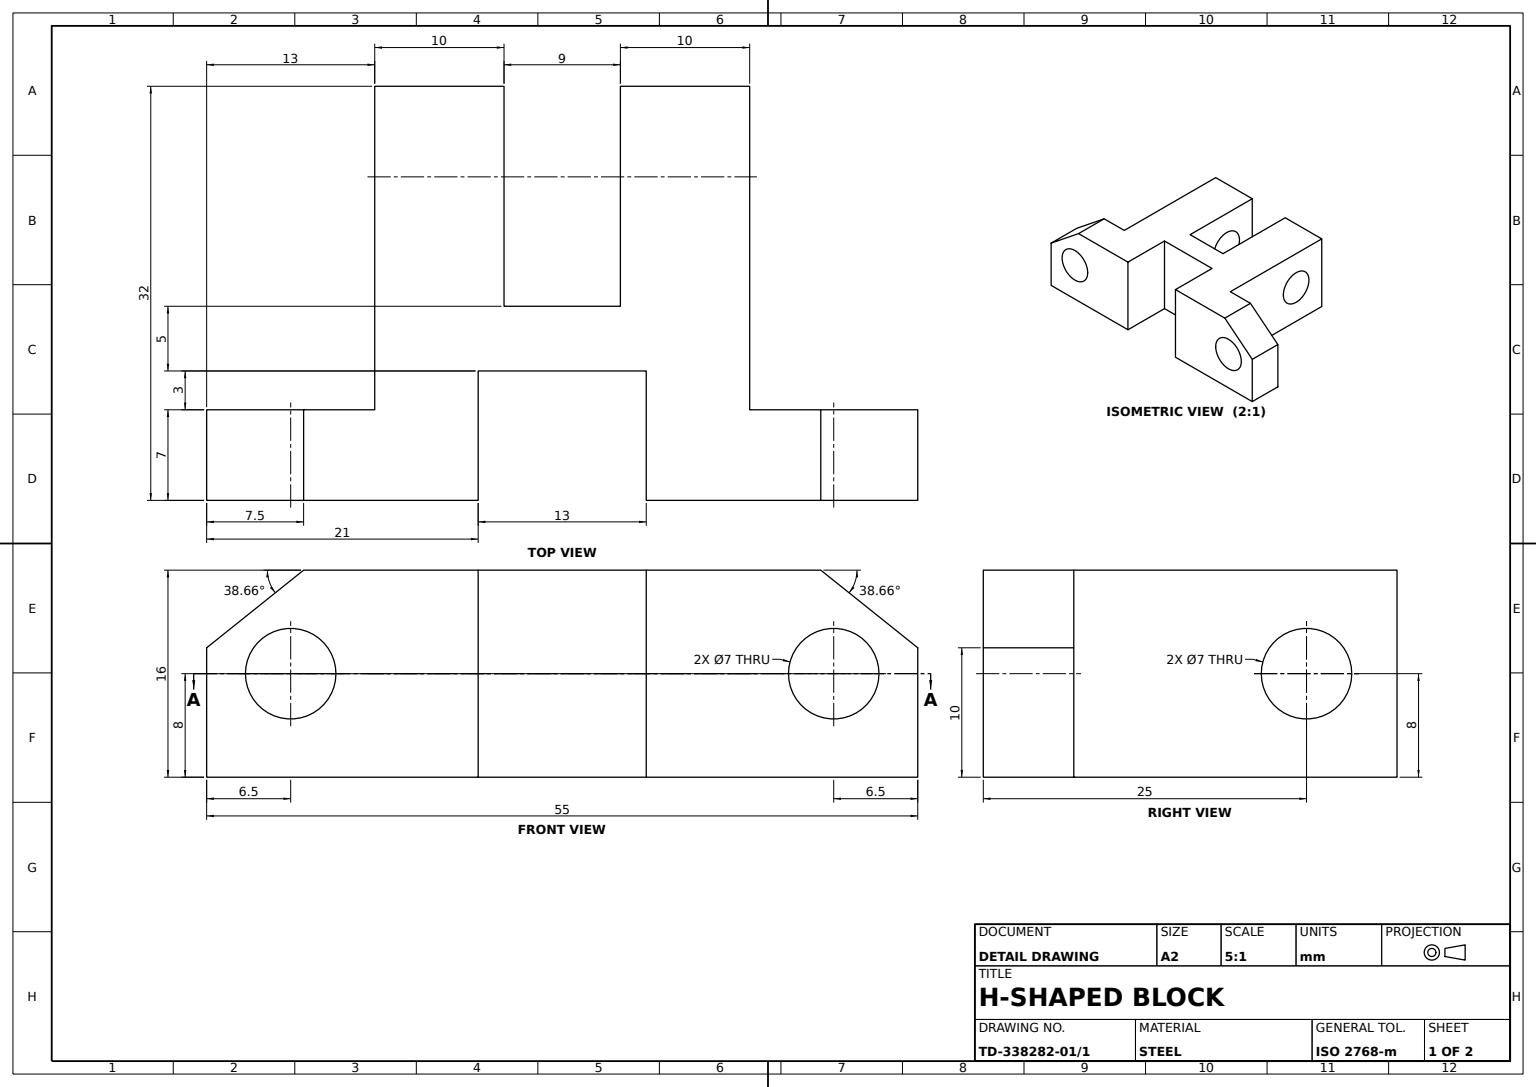
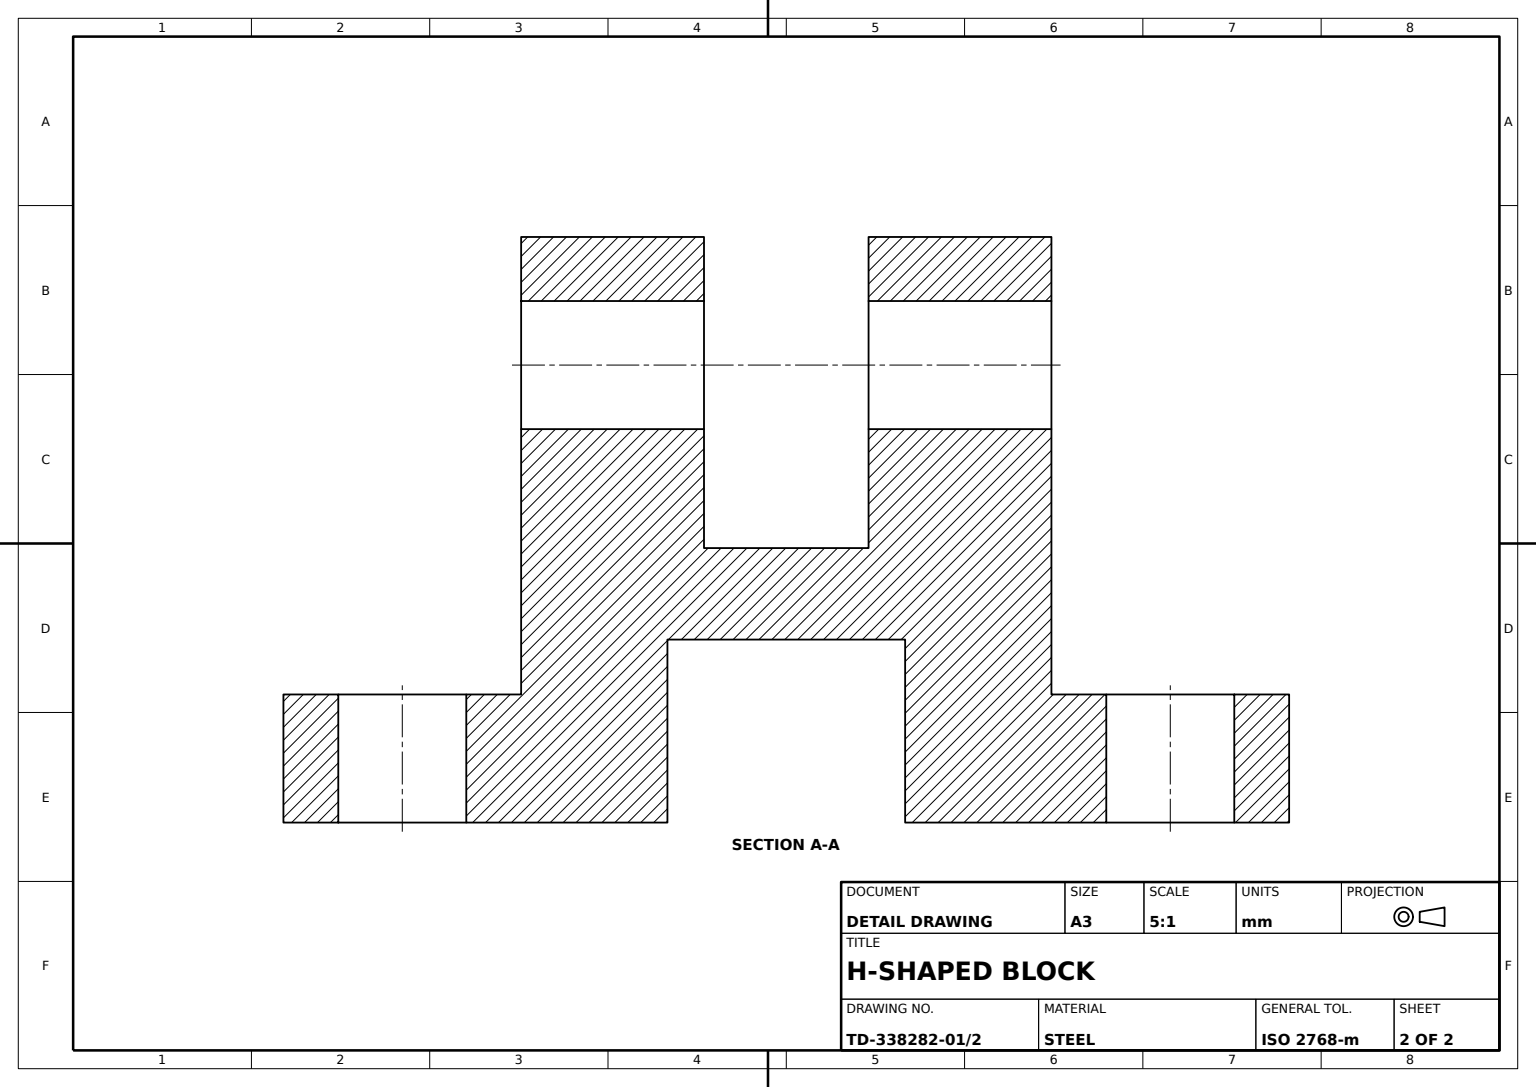
SolidWorks part; units mm, degrees
material "Plain Carbon Steel"
ref_plane "Front Plane" through (0, 0, 0) normal (0, 0, 1) x (1, 0, 0)
ref_plane "Top Plane" through (0, 0, 0) normal (0, 1, 0) x (1, 0, 0)
ref_plane "Right Plane" through (0, 0, 0) normal (1, 0, 0) x (0, 0, -1)
sketch "Base Block Profile" plane through (0, 0, 0) normal (0, 0, 1) x (1, 0, 0)
  line L1 (-27.5, 8) -> (27.5, 8)
  line L2 (-27.5, 8) -> (-27.5, -8)
  line L3 (-27.5, -8) -> (27.5, -8)
  line L4 (27.5, 8) -> (27.5, -8)
  line L5 (-27.5, 8) -> (27.5, -8) construction
  line L6 (-27.5, -8) -> (27.5, 8) construction
  point P0 (0, 0)
  dimension "D1" = 55
  dimension "D2" = 16
extrude "Base Block" add sketch "Base Block Profile" along normal blind 32 contours L2 L1 L4 L3
sketch "Centre Notch Profile" plane through (0, 8, 0) normal (0, 1, 0) x (1, 0, 0)
  line L0 (0, 0) -> (0, -13.9137) construction
  line L2 (-27.5, 0) -> (-14.5, 0)
  line L3 (-27.5, 0) -> (-27.5, -25)
  line L4 (-27.5, -25) -> (-14.5, -25)
  line L5 (-14.5, 0) -> (-14.5, -25)
  line L6 (27.5, -25) -> (14.5, -25)
  line L7 (14.5, 0) -> (14.5, -25)
  line L8 (27.5, 0) -> (14.5, 0)
  line L9 (27.5, 0) -> (27.5, -25)
  dimension "D1" = 13
  dimension "D2" = 25
extrude "Centre Notch" cut sketch "Centre Notch Profile" against normal through all both and the other way through all
sketch "Side Step Cut Profile" plane through (0, 8, 0) normal (0, 1, 0) x (1, 0, 0)
  line L0 (0, 0) -> (0, -32) construction
  line L2 (-27.5, -32) -> (27.5, -32) construction
  line L4 (-6.5, -32) -> (6.5, -32)
  line L5 (-6.5, -32) -> (-6.5, -22)
  line L6 (-6.5, -22) -> (6.5, -22)
  line L7 (6.5, -32) -> (6.5, -22)
  dimension "D1" = 13
  dimension "D2" = 6.5
  dimension "D3" = 10
extrude "Side Step Cut" cut sketch "Side Step Cut Profile" against normal through all both
sketch "Corner Bevel Profile" plane through (0, 8, 0) normal (0, 1, 0) x (1, 0, 0)
  line L0 (-14.5, 0) -> (14.5, 0) construction
  line L1 (-4.5, 0) -> (4.5, 0)
  line L2 (-4.5, 0) -> (-4.5, -17)
  line L3 (-4.5, -17) -> (4.5, -17)
  line L4 (4.5, 0) -> (4.5, -17)
  line L5 (6.5, -22) -> (-6.5, -22) construction
  dimension "D1" = 9
  dimension "D2" = 5
  dimension "D3" = 4.5
extrude "Corner Bevel Cut" cut sketch "Corner Bevel Profile" against normal through all both
sketch "Lug Slot Profile" plane through (0, 0, 25) normal (0, 0, -1) x (-1, 0, 0)
  line L0 (27.5, -8) -> (27.5, 2)
  line L2 (27.5, 2) -> (20, 8)
  line L4 (20, 8) -> (-20, 8)
  line L6 (-20, 8) -> (-27.5, 2)
  line L8 (-27.5, 2) -> (-27.5, 8)
  line L9 (-27.5, 8) -> (-20, 8)
  line L10 (27.5, 2) -> (27.5, 8)
  line L11 (27.5, 8) -> (20, 8)
  line L12 (27.5, 2) -> (27.5, 8)
  line L13 (20, 8) -> (27.5, 8)
  line L14 (20, 8) -> (28.3076, 8)
  line L15 (28.3076, 8) -> (28.3076, 2)
  line L16 (28.3076, 2) -> (27.5, 2)
  line L17 (14.5, -8) -> (14.5, 8) construction
  line M1 (27.5, 8) -> (14.5, 8)
  line M4 (27.5, -8) -> (27.5, 8)
  dimension "D1" = 10
  dimension "D2" = 10
  dimension "D3" = 40
  dimension "D4" = 20
  dimension "D5" = 13.8076
  dimension "D6" = 7.5
  dimension "D7" = 42
  dimension "D8" = 16
extrude "Lug Slot Cut" cut sketch "Lug Slot Profile" against normal through all both contours L9 L8 L6 | L2 M4 M1
sketch "Lug Holes Ø7 Sketch" plane through (0, 0, 25) normal (0, 0, -1) x (-1, 0, 0)
  line L0 (14.5, 0) -> (27.5, 0)
  line L1 (14.5, -8) -> (14.5, 8) construction
  line L2 (14.5, -8) -> (14.5, 8)
  line L3 (27.5, -8) -> (27.5, 2) construction
  line L4 (27.5, -8) -> (27.5, 2)
  line L5 (0, 0) -> (0, -15.0467) construction
  circle A0 centre (21, 0) radius 3.5
  circle A1 centre (-21, 0) radius 3.5
  dimension "D1" = 7
extrude "Lug Holes Ø7" cut sketch "Lug Holes Ø7 Sketch" against normal through all both contours L0 A0 | L0 A0 | A1
sketch "Cross Hole Ø7 Sketch" plane through (14.5, 0, 0) normal (1, 0, 0) x (0, 0, -1)
  line L0 (0, 0) -> (-7, 0)
  line L1 (0, -8) -> (0, 8) construction
  circle A0 centre (-7, 0) radius 3.5
  dimension "D2" = 7
  dimension "D1" = 7
extrude "Cross Hole Ø7" cut sketch "Cross Hole Ø7 Sketch" against normal through all both
